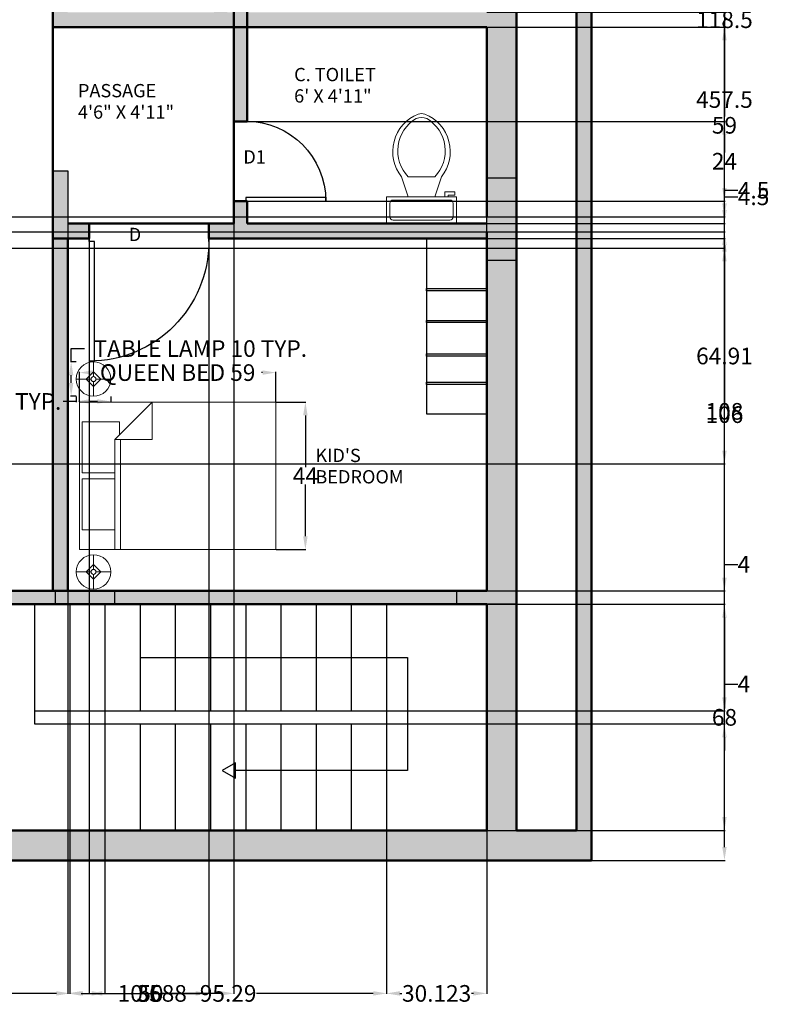
# Model space of a CAD drawing. Units: inches. Extents: x -12 to 887, y 330 to 874.
# Tile 6 of 9: x 662 to 887, y 330 to 626. Entities that reach past the tile are written whole.
import ezdxf

# ---------------------------------------------------------------- set-up
doc = ezdxf.new("R2010")
doc.units = ezdxf.units.IN
doc.header["$MEASUREMENT"] = 0
for name, color, linetype, lineweight in [('A-ANNO-DIMS', 2, 'Continuous', 18), ('A-ANNO-TEXT', 3, 'Continuous', 18), ('A-AREA-IDEN', 7, 'Continuous', 18), ('A-DOOR', 4, 'Continuous', 25), ('A-FLOR-FIXT', 8, 'Continuous', 18), ('A-FLOR-STRS', 3, 'Continuous', 25), ('A-FURN', 9, 'Continuous', 18), ('A-GLAZ', 4, 'Continuous', 25), ('A-WALL', 7, 'Continuous', 50), ('A-WALL-PATT', 5, 'Continuous', 13)]:
    doc.layers.add(name, color=color, linetype=linetype, lineweight=lineweight)
doc.styles.get("Standard").update_dxf_attribs({"font": 'arial.ttf'})
doc.dimstyles.get("Standard").update_dxf_attribs({"dimtxt": 5, "dimasz": 4, "dimexe": 0.18, "dimexo": 0.0625, "dimgap": 0.09, "dimtad": 0, "dimtih": 1, "dimtoh": 1, "dimdec": 1, "dimzin": 0, "dimdsep": 46, "dimlunit": 4, "dimtxsty": 'Standard', "dimcen": 0.09, "dimadec": 0, "dimazin": 0, "dimtfac": 1, "dimtdec": 1, "dimtofl": 0, "dimtmove": 0, "dimatfit": 3, "dimfxl": 1, "dimtolj": 1, "dimtzin": 0, "dimarcsym": 0})

# ---------------------------------------------------------------- blocks, each defined once
blk = doc.blocks.new('*U5')
for p, q in [((0, 0), (0, -6)), ((40, 0), (40, -6))]:
    blk.add_line(p, q)
blk.add_lwpolyline([(0, 0), (0, 40), (1.75, 40), (1.75, 0)], close=True)
blk.add_arc((0, 0), 40, 0, 90)
blk = doc.blocks.new('Bed - Queen')
for p, q in [((0, -80.00003), (0, 0)), ((0, 0), (59.99999, 0)), ((59.99999, 0), (59.99999, -80.00003)), ((7.99999, -1.2), (28.79998, -1.2)), ((7.99999, -14.4), (7.99999, -1.2)), ((28.79998, -1.2), (28.79998, -14.4)), ((31.19999, -1.2), (51.99999, -1.2)), ((31.19999, -14.4), (31.19999, -1.2)), ((51.99999, -1.2), (51.99999, -16.4)), ((0, -14.4), (44.8, -14.4)), ((59.99999, -29.6), (44.8, -14.4)), ((44.8, -14.4), (44.8, -29.6)), ((44.8, -16.8), (0, -16.8)), ((51.99999, -16.4), (46.79936, -16.4)), ((44.8, -29.6), (59.99999, -29.6)), ((59.99999, -80.00003), (0, -80.00003))]:
    blk.add_line(p, q)
blk = doc.blocks.new('Lamp - Table')
for p, q in [((0, 7), (0, 1)), ((-1, 0), (-7, 0)), ((0, 3), (-3, 0)), ((-3, 0), (0, -3)), ((3, 0), (0, 3)), ((0, -3), (3, 0)), ((1, 0), (7, 0)), ((0, -1), (0, -7))]:
    blk.add_line(p, q)
for radius in [7, 1]:
    blk.add_circle((0, 0), radius)
blk = doc.blocks.new('*U12')
for p, q in [((241.3, -152.4), (241.3, -50.8)), ((-254, -215.9), (-203.2, -215.9)), ((-254, -241.3), (-254, -215.9)), ((-203.2, -215.9), (-203.2, -203.2)), ((-177.8, -203.2), (-177.8, -241.3)), ((-101.6, -203.2), (-152.4, -355.6)), ((101.6, -203.2), (152.4, -355.6)), ((-177.8, -241.3), (-254, -241.3)), ((101.6, -355.6), (-101.6, -355.6))]:
    blk.add_line(p, q)
blk.add_lwpolyline([(266.7, -203.2), (266.7, 0), (-266.7, 0), (-266.7, -203.2)], close=True)
for points in [[(-241.3, -50.8), (-241.3, -152.4)], [(215.9, -25.4), (-215.9, -25.4)], [(-215.9, -177.8), (215.9, -177.8)]]:
    blk.add_lwpolyline(points)
for centre, radius, start, end in [((-219.1, -47.6), 22.5, 81.8699, 188.1301), ((219.1, -47.6), 22.5, 351.8699, 98.1301), ((-219.1, -155.6), 22.5, 171.8699, 278.1301), ((219.1, -155.6), 22.5, 261.8699, 8.1301), ((89.4, -548.1), 309.1, 141.46911, 247.97143), ((106.7, -554.2), 287.8, 136.36773, 238.94682), ((-89.4, -548.1), 309.1, 292.02843, 38.53071), ((-106.7, -554.2), 287.8, 301.05301, 43.63209), ((0, -708.1), 101.6, 245.73182, 294.26817), ((0, -736.6), 101.6, 254.86053, 285.13947)]:
    blk.add_arc(centre, radius, start, end)
blk = doc.blocks.new('*D18')
at = {"layer": 'A-ANNO-DIMS', "color": 0, "lineweight": -2, "transparency": 16777216}
for p, q in [((677.1, 523.03), (677.1, 527.03)), ((677.1, 527.03), (681.1, 527.03)), ((678.58, 523.03), (676.92, 523.03)), ((677.1, 516.69), (677.1, 519.03)), ((678.58, 512.69), (676.92, 512.69))]:
    blk.add_line(p, q, dxfattribs=at)
at = {"layer": 'A-ANNO-DIMS', "color": 0, "transparency": 16777216}
for points in [[(676.43, 519.03), (677.76, 519.03), (677.1, 523.03)], [(676.43, 516.69), (677.76, 516.69), (677.1, 512.69)]]:
    blk.add_solid(points, dxfattribs=at)
at = {"layer": 'Defpoints', "color": 0, "transparency": 16777216}
for p in [(677.1, 523.03), (678.65, 523.03), (678.65, 512.69)]:
    blk.add_point(p, dxfattribs=at)
at = {"layer": 'A-ANNO-DIMS', "color": 0, "transparency": 16777216, "insert": (715.93, 527.03), "char_height": 5, "attachment_point": 5}
blk.add_mtext('\\A1;TABLE LAMP 10 TYP.', dxfattribs=at)
blk = doc.blocks.new('*D19')
at = {"layer": 'A-ANNO-DIMS', "color": 0, "lineweight": -2, "transparency": 16777216}
for p, q in [((678.65, 512.63), (678.65, 510.96)), ((688.99, 512.63), (688.99, 510.96)), ((678.65, 511.14), (674.65, 511.14)), ((684.99, 511.14), (682.65, 511.14))]:
    blk.add_line(p, q, dxfattribs=at)
at = {"layer": 'A-ANNO-DIMS', "color": 0, "transparency": 16777216}
for points in [[(682.65, 511.8), (682.65, 510.47), (678.65, 511.14)], [(684.99, 511.8), (684.99, 510.47), (688.99, 511.14)]]:
    blk.add_solid(points, dxfattribs=at)
at = {"layer": 'Defpoints', "color": 0, "transparency": 16777216}
for p in [(678.65, 512.69), (688.99, 512.69), (678.65, 511.14)]:
    blk.add_point(p, dxfattribs=at)
at = {"layer": 'A-ANNO-DIMS', "color": 0, "transparency": 16777216, "insert": (662.62, 511.14), "char_height": 5, "attachment_point": 5}
blk.add_mtext('\\A1;10 TYP.', dxfattribs=at)
blk = doc.blocks.new('*D22')
at = {"layer": 'A-ANNO-DIMS', "color": 0, "lineweight": -2, "transparency": 16777216}
for p, q in [((679.56, 511.01), (679.56, 519.99)), ((683.56, 519.81), (683.91, 519.81)), ((734.67, 519.81), (734.33, 519.81)), ((738.67, 511.01), (738.67, 519.99))]:
    blk.add_line(p, q, dxfattribs=at)
at = {"layer": 'A-ANNO-DIMS', "color": 0, "transparency": 16777216}
for points in [[(683.56, 520.48), (683.56, 519.14), (679.56, 519.81)], [(734.67, 520.48), (734.67, 519.14), (738.67, 519.81)]]:
    blk.add_solid(points, dxfattribs=at)
at = {"layer": 'Defpoints', "color": 0, "transparency": 16777216}
for p in [(679.56, 519.81), (679.56, 510.94), (738.67, 510.94)]:
    blk.add_point(p, dxfattribs=at)
at = {"layer": 'A-ANNO-DIMS', "color": 0, "transparency": 16777216, "insert": (709.12, 519.81), "char_height": 5, "attachment_point": 5}
blk.add_mtext('\\A1;QUEEN BED 59', dxfattribs=at)
blk = doc.blocks.new('*D23')
at = {"layer": 'A-ANNO-DIMS', "color": 0, "lineweight": -2, "transparency": 16777216}
for p, q in [((738.74, 510.94), (747.72, 510.94)), ((747.54, 506.94), (747.54, 491.37)), ((747.54, 470.61), (747.54, 486.19)), ((738.74, 466.61), (747.72, 466.61))]:
    blk.add_line(p, q, dxfattribs=at)
at = {"layer": 'A-ANNO-DIMS', "color": 0, "transparency": 16777216}
for points in [[(746.87, 506.94), (748.21, 506.94), (747.54, 510.94)], [(746.87, 470.61), (748.21, 470.61), (747.54, 466.61)]]:
    blk.add_solid(points, dxfattribs=at)
at = {"layer": 'Defpoints', "color": 0, "transparency": 16777216}
for p in [(738.67, 510.94), (747.54, 510.94), (738.67, 466.61)]:
    blk.add_point(p, dxfattribs=at)
at = {"layer": 'A-ANNO-DIMS', "color": 0, "transparency": 16777216, "insert": (747.54, 488.78), "char_height": 5, "attachment_point": 5}
blk.add_mtext('\\A1;44', dxfattribs=at)
blk = doc.blocks.new('*D60')
at = {"layer": 'A-ANNO-DIMS', "color": 0, "lineweight": -2, "transparency": 16777216}
for p, q in [((383.99, 450.16), (873.75, 450.16)), ((873.57, 446.16), (873.57, 418.8)), ((873.57, 386.16), (873.57, 413.52)), ((383.99, 382.16), (873.75, 382.16))]:
    blk.add_line(p, q, dxfattribs=at)
at = {"layer": 'A-ANNO-DIMS', "color": 0, "transparency": 16777216}
for points in [[(872.9, 446.16), (874.24, 446.16), (873.57, 450.16)], [(872.9, 386.16), (874.24, 386.16), (873.57, 382.16)]]:
    blk.add_solid(points, dxfattribs=at)
at = {"layer": 'Defpoints', "color": 0, "transparency": 16777216}
for p in [(383.93, 450.16), (873.57, 450.16), (383.93, 382.16)]:
    blk.add_point(p, dxfattribs=at)
at = {"layer": 'A-ANNO-DIMS', "color": 0, "transparency": 16777216, "insert": (873.57, 416.16), "char_height": 5, "attachment_point": 5}
blk.add_mtext('\\A1;68', dxfattribs=at)
blk = doc.blocks.new('*D61')
at = {"layer": 'A-ANNO-DIMS', "color": 0, "lineweight": -2, "transparency": 16777216}
for p, q in [((873.57, 458.16), (873.57, 462.16)), ((873.57, 462.16), (877.57, 462.16)), ((383.99, 454.16), (873.75, 454.16)), ((383.99, 450.16), (873.75, 450.16)), ((873.57, 446.16), (873.57, 442.16))]:
    blk.add_line(p, q, dxfattribs=at)
at = {"layer": 'A-ANNO-DIMS', "color": 0, "transparency": 16777216}
for points in [[(872.9, 458.16), (874.24, 458.16), (873.57, 454.16)], [(872.9, 446.16), (874.24, 446.16), (873.57, 450.16)]]:
    blk.add_solid(points, dxfattribs=at)
at = {"layer": 'Defpoints', "color": 0, "transparency": 16777216}
for p in [(383.93, 454.16), (873.57, 454.16), (383.93, 450.16)]:
    blk.add_point(p, dxfattribs=at)
at = {"layer": 'A-ANNO-DIMS', "color": 0, "transparency": 16777216, "insert": (879.39, 462.16), "char_height": 5, "attachment_point": 5}
blk.add_mtext('\\A1;4', dxfattribs=at)
blk = doc.blocks.new('*D62')
at = {"layer": 'A-ANNO-DIMS', "color": 0, "lineweight": -2, "transparency": 16777216}
for p, q in [((383.99, 562.16), (873.75, 562.16)), ((873.57, 558.16), (873.57, 510.8)), ((873.57, 458.16), (873.57, 505.52)), ((383.99, 454.16), (873.75, 454.16))]:
    blk.add_line(p, q, dxfattribs=at)
at = {"layer": 'A-ANNO-DIMS', "color": 0, "transparency": 16777216}
for points in [[(872.9, 558.16), (874.24, 558.16), (873.57, 562.16)], [(872.9, 458.16), (874.24, 458.16), (873.57, 454.16)]]:
    blk.add_solid(points, dxfattribs=at)
at = {"layer": 'Defpoints', "color": 0, "transparency": 16777216}
for p in [(383.93, 562.16), (873.57, 562.16), (383.93, 454.16)]:
    blk.add_point(p, dxfattribs=at)
at = {"layer": 'A-ANNO-DIMS', "color": 0, "transparency": 16777216, "insert": (873.57, 508.16), "char_height": 5, "attachment_point": 5}
blk.add_mtext('\\A1;108', dxfattribs=at)
blk = doc.blocks.new('*D63')
at = {"layer": 'A-ANNO-DIMS', "color": 0, "lineweight": -2, "transparency": 16777216}
for p, q in [((873.57, 570.66), (873.57, 574.66)), ((873.57, 574.66), (877.57, 574.66)), ((383.99, 566.66), (873.75, 566.66)), ((383.99, 562.16), (873.75, 562.16)), ((873.57, 558.16), (873.57, 554.16))]:
    blk.add_line(p, q, dxfattribs=at)
at = {"layer": 'A-ANNO-DIMS', "color": 0, "transparency": 16777216}
for points in [[(872.9, 570.66), (874.24, 570.66), (873.57, 566.66)], [(872.9, 558.16), (874.24, 558.16), (873.57, 562.16)]]:
    blk.add_solid(points, dxfattribs=at)
at = {"layer": 'Defpoints', "color": 0, "transparency": 16777216}
for p in [(383.93, 566.66), (873.57, 566.66), (383.93, 562.16)]:
    blk.add_point(p, dxfattribs=at)
at = {"layer": 'A-ANNO-DIMS', "color": 0, "transparency": 16777216, "insert": (882.33, 574.66), "char_height": 5, "attachment_point": 5}
blk.add_mtext('\\A1;4.5', dxfattribs=at)
blk = doc.blocks.new('*D64')
at = {"layer": 'A-ANNO-DIMS', "color": 0, "lineweight": -2, "transparency": 16777216}
for p, q in [((383.99, 685.16), (873.75, 685.16)), ((873.57, 681.16), (873.57, 628.55)), ((873.57, 570.66), (873.57, 623.27)), ((383.99, 566.66), (873.75, 566.66))]:
    blk.add_line(p, q, dxfattribs=at)
at = {"layer": 'A-ANNO-DIMS', "color": 0, "transparency": 16777216}
for points in [[(872.9, 681.16), (874.24, 681.16), (873.57, 685.16)], [(872.9, 570.66), (874.24, 570.66), (873.57, 566.66)]]:
    blk.add_solid(points, dxfattribs=at)
at = {"layer": 'Defpoints', "color": 0, "transparency": 16777216}
for p in [(383.93, 685.16), (873.57, 685.16), (383.93, 566.66)]:
    blk.add_point(p, dxfattribs=at)
at = {"layer": 'A-ANNO-DIMS', "color": 0, "transparency": 16777216, "insert": (873.57, 625.91), "char_height": 5, "attachment_point": 5}
blk.add_mtext('\\A1;118.5', dxfattribs=at)
blk = doc.blocks.new('*D95')
at = {"layer": 'A-ANNO-DIMS', "color": 0, "lineweight": -2, "transparency": 16777216}
for p, q in [((493.07, 382.1), (493.07, 332.98)), ((676.66, 382.1), (676.66, 332.98)), ((497.07, 333.16), (576.57, 333.16)), ((672.66, 333.16), (593.15, 333.16))]:
    blk.add_line(p, q, dxfattribs=at)
at = {"layer": 'A-ANNO-DIMS', "color": 0, "transparency": 16777216}
for points in [[(497.07, 333.83), (497.07, 332.49), (493.07, 333.16)], [(672.66, 333.83), (672.66, 332.49), (676.66, 333.16)]]:
    blk.add_solid(points, dxfattribs=at)
at = {"layer": 'Defpoints', "color": 0, "transparency": 16777216}
for p in [(493.07, 382.16), (676.66, 382.16), (676.66, 333.16)]:
    blk.add_point(p, dxfattribs=at)
at = {"layer": 'A-ANNO-DIMS', "color": 0, "transparency": 16777216, "insert": (584.86, 333.16), "char_height": 5, "attachment_point": 5}
blk.add_mtext('\\A1;183.6', dxfattribs=at)
blk = doc.blocks.new('*D96')
at = {"layer": 'A-ANNO-DIMS', "color": 0, "lineweight": -2, "transparency": 16777216}
for p, q in [((676.66, 382.1), (676.66, 332.98)), ((771.95, 382.1), (771.95, 332.98)), ((680.66, 333.16), (715.77, 333.16)), ((767.95, 333.16), (732.83, 333.16))]:
    blk.add_line(p, q, dxfattribs=at)
at = {"layer": 'A-ANNO-DIMS', "color": 0, "transparency": 16777216}
for points in [[(680.66, 333.83), (680.66, 332.49), (676.66, 333.16)], [(767.95, 333.83), (767.95, 332.49), (771.95, 333.16)]]:
    blk.add_solid(points, dxfattribs=at)
at = {"layer": 'Defpoints', "color": 0, "transparency": 16777216}
for p in [(676.66, 382.16), (771.95, 382.16), (771.95, 333.16)]:
    blk.add_point(p, dxfattribs=at)
at = {"layer": 'A-ANNO-DIMS', "color": 0, "transparency": 16777216, "insert": (724.3, 333.16), "char_height": 5, "attachment_point": 5}
blk.add_mtext('\\A1;95.29', dxfattribs=at)
blk = doc.blocks.new('*D97')
at = {"layer": 'A-ANNO-DIMS', "color": 0, "lineweight": -2, "transparency": 16777216}
for p, q in [((771.95, 382.1), (771.95, 332.98)), ((802.07, 382.1), (802.07, 332.98)), ((775.95, 333.16), (776.54, 333.16)), ((798.07, 333.16), (797.47, 333.16))]:
    blk.add_line(p, q, dxfattribs=at)
at = {"layer": 'A-ANNO-DIMS', "color": 0, "transparency": 16777216}
for points in [[(775.95, 333.83), (775.95, 332.49), (771.95, 333.16)], [(798.07, 333.83), (798.07, 332.49), (802.07, 333.16)]]:
    blk.add_solid(points, dxfattribs=at)
at = {"layer": 'Defpoints', "color": 0, "transparency": 16777216}
for p in [(771.95, 382.16), (802.07, 382.16), (802.07, 333.16)]:
    blk.add_point(p, dxfattribs=at)
at = {"layer": 'A-ANNO-DIMS', "color": 0, "transparency": 16777216, "insert": (787.01, 333.16), "char_height": 5, "attachment_point": 5}
blk.add_mtext('\\A1;30.123', dxfattribs=at)
blk = doc.blocks.new('*D98')
at = {"layer": 'A-ANNO-DIMS', "color": 0, "lineweight": -2, "transparency": 16777216}
for p, q in [((460.13, 830.66), (873.75, 830.66)), ((873.57, 826.66), (873.57, 604.54)), ((873.57, 377.16), (873.57, 599.28)), ((460.13, 373.16), (873.75, 373.16))]:
    blk.add_line(p, q, dxfattribs=at)
at = {"layer": 'A-ANNO-DIMS', "color": 0, "transparency": 16777216}
for points in [[(872.9, 826.66), (874.24, 826.66), (873.57, 830.66)], [(872.9, 377.16), (874.24, 377.16), (873.57, 373.16)]]:
    blk.add_solid(points, dxfattribs=at)
at = {"layer": 'Defpoints', "color": 0, "transparency": 16777216}
for p in [(460.07, 830.66), (873.57, 830.66), (460.07, 373.16)]:
    blk.add_point(p, dxfattribs=at)
at = {"layer": 'A-ANNO-DIMS', "color": 0, "transparency": 16777216, "insert": (873.57, 601.91), "char_height": 5, "attachment_point": 5}
blk.add_mtext('\\A1;457.5', dxfattribs=at)
blk = doc.blocks.new('*D104')
at = {"layer": 'A-ANNO-DIMS', "color": 0, "lineweight": -2, "transparency": 16777216}
for p, q in [((802.13, 450.16), (873.75, 450.16)), ((873.57, 446.16), (873.57, 418.8)), ((873.57, 386.16), (873.57, 413.52)), ((802.13, 382.16), (873.75, 382.16))]:
    blk.add_line(p, q, dxfattribs=at)
at = {"layer": 'A-ANNO-DIMS', "color": 0, "transparency": 16777216}
for points in [[(872.9, 446.16), (874.24, 446.16), (873.57, 450.16)], [(872.9, 386.16), (874.24, 386.16), (873.57, 382.16)]]:
    blk.add_solid(points, dxfattribs=at)
at = {"layer": 'Defpoints', "color": 0, "transparency": 16777216}
for p in [(802.07, 450.16), (873.57, 450.16), (802.07, 382.16)]:
    blk.add_point(p, dxfattribs=at)
at = {"layer": 'A-ANNO-DIMS', "color": 0, "transparency": 16777216, "insert": (873.57, 416.16), "char_height": 5, "attachment_point": 5}
blk.add_mtext('\\A1;68', dxfattribs=at)
blk = doc.blocks.new('*D105')
at = {"layer": 'A-ANNO-DIMS', "color": 0, "lineweight": -2, "transparency": 16777216}
for p, q in [((873.57, 458.16), (873.57, 462.16)), ((873.57, 462.16), (877.57, 462.16)), ((802.13, 454.16), (873.75, 454.16)), ((802.13, 450.16), (873.75, 450.16)), ((873.57, 446.16), (873.57, 442.16))]:
    blk.add_line(p, q, dxfattribs=at)
at = {"layer": 'A-ANNO-DIMS', "color": 0, "transparency": 16777216}
for points in [[(872.9, 458.16), (874.24, 458.16), (873.57, 454.16)], [(872.9, 446.16), (874.24, 446.16), (873.57, 450.16)]]:
    blk.add_solid(points, dxfattribs=at)
at = {"layer": 'Defpoints', "color": 0, "transparency": 16777216}
for p in [(802.07, 454.16), (873.57, 454.16), (802.07, 450.16)]:
    blk.add_point(p, dxfattribs=at)
at = {"layer": 'A-ANNO-DIMS', "color": 0, "transparency": 16777216, "insert": (879.39, 462.16), "char_height": 5, "attachment_point": 5}
blk.add_mtext('\\A1;4', dxfattribs=at)
blk = doc.blocks.new('*D106')
at = {"layer": 'A-ANNO-DIMS', "color": 0, "lineweight": -2, "transparency": 16777216}
for p, q in [((802.13, 560.16), (873.75, 560.16)), ((873.57, 556.16), (873.57, 509.8)), ((873.57, 458.16), (873.57, 504.52)), ((802.13, 454.16), (873.75, 454.16))]:
    blk.add_line(p, q, dxfattribs=at)
at = {"layer": 'A-ANNO-DIMS', "color": 0, "transparency": 16777216}
for points in [[(872.9, 556.16), (874.24, 556.16), (873.57, 560.16)], [(872.9, 458.16), (874.24, 458.16), (873.57, 454.16)]]:
    blk.add_solid(points, dxfattribs=at)
at = {"layer": 'Defpoints', "color": 0, "transparency": 16777216}
for p in [(802.07, 560.16), (873.57, 560.16), (802.07, 454.16)]:
    blk.add_point(p, dxfattribs=at)
at = {"layer": 'A-ANNO-DIMS', "color": 0, "transparency": 16777216, "insert": (873.57, 507.16), "char_height": 5, "attachment_point": 5}
blk.add_mtext('\\A1;106', dxfattribs=at)
blk = doc.blocks.new('*D107')
at = {"layer": 'A-ANNO-DIMS', "color": 0, "lineweight": -2, "transparency": 16777216}
for p, q in [((873.57, 568.66), (873.57, 572.66)), ((873.57, 572.66), (877.57, 572.66)), ((802.13, 564.66), (873.75, 564.66)), ((802.13, 560.16), (873.75, 560.16)), ((873.57, 556.16), (873.57, 552.16))]:
    blk.add_line(p, q, dxfattribs=at)
at = {"layer": 'A-ANNO-DIMS', "color": 0, "transparency": 16777216}
for points in [[(872.9, 568.66), (874.24, 568.66), (873.57, 564.66)], [(872.9, 556.16), (874.24, 556.16), (873.57, 560.16)]]:
    blk.add_solid(points, dxfattribs=at)
at = {"layer": 'Defpoints', "color": 0, "transparency": 16777216}
for p in [(802.07, 564.66), (873.57, 564.66), (802.07, 560.16)]:
    blk.add_point(p, dxfattribs=at)
at = {"layer": 'A-ANNO-DIMS', "color": 0, "transparency": 16777216, "insert": (882.33, 572.66), "char_height": 5, "attachment_point": 5}
blk.add_mtext('\\A1;4.5', dxfattribs=at)
blk = doc.blocks.new('*D108')
at = {"layer": 'A-ANNO-DIMS', "color": 0, "lineweight": -2, "transparency": 16777216}
for p, q in [((802.13, 623.66), (873.75, 623.66)), ((873.57, 619.66), (873.57, 596.8)), ((873.57, 568.66), (873.57, 591.52)), ((802.13, 564.66), (873.75, 564.66))]:
    blk.add_line(p, q, dxfattribs=at)
at = {"layer": 'A-ANNO-DIMS', "color": 0, "transparency": 16777216}
for points in [[(872.9, 619.66), (874.24, 619.66), (873.57, 623.66)], [(872.9, 568.66), (874.24, 568.66), (873.57, 564.66)]]:
    blk.add_solid(points, dxfattribs=at)
at = {"layer": 'Defpoints', "color": 0, "transparency": 16777216}
for p in [(802.07, 623.66), (873.57, 623.66), (802.07, 564.66)]:
    blk.add_point(p, dxfattribs=at)
at = {"layer": 'A-ANNO-DIMS', "color": 0, "transparency": 16777216, "insert": (873.57, 594.16), "char_height": 5, "attachment_point": 5}
blk.add_mtext('\\A1;59', dxfattribs=at)
blk = doc.blocks.new('*D109')
at = {"layer": 'A-ANNO-DIMS', "color": 0, "lineweight": -2, "transparency": 16777216}
for p, q in [((873.57, 632.16), (873.57, 636.16)), ((873.57, 636.16), (877.57, 636.16)), ((802.13, 628.16), (873.75, 628.16)), ((802.13, 623.66), (873.75, 623.66)), ((873.57, 619.66), (873.57, 615.66))]:
    blk.add_line(p, q, dxfattribs=at)
at = {"layer": 'A-ANNO-DIMS', "color": 0, "transparency": 16777216}
for points in [[(872.9, 632.16), (874.24, 632.16), (873.57, 628.16)], [(872.9, 619.66), (874.24, 619.66), (873.57, 623.66)]]:
    blk.add_solid(points, dxfattribs=at)
at = {"layer": 'Defpoints', "color": 0, "transparency": 16777216}
for p in [(802.07, 628.16), (873.57, 628.16), (802.07, 623.66)]:
    blk.add_point(p, dxfattribs=at)
at = {"layer": 'A-ANNO-DIMS', "color": 0, "transparency": 16777216, "insert": (882.33, 636.16), "char_height": 5, "attachment_point": 5}
blk.add_mtext('\\A1;4.5', dxfattribs=at)
blk = doc.blocks.new('*D115')
at = {"layer": 'A-ANNO-DIMS', "color": 0, "lineweight": -2, "transparency": 16777216}
for p, q in [((676.07, 564.6), (676.07, 332.98)), ((726.07, 564.6), (726.07, 332.98)), ((680.07, 333.16), (697.41, 333.16)), ((722.07, 333.16), (704.73, 333.16))]:
    blk.add_line(p, q, dxfattribs=at)
at = {"layer": 'A-ANNO-DIMS', "color": 0, "transparency": 16777216}
for points in [[(680.07, 333.83), (680.07, 332.49), (676.07, 333.16)], [(722.07, 333.83), (722.07, 332.49), (726.07, 333.16)]]:
    blk.add_solid(points, dxfattribs=at)
at = {"layer": 'Defpoints', "color": 0, "transparency": 16777216}
for p in [(676.07, 564.66), (726.07, 564.66), (726.07, 333.16)]:
    blk.add_point(p, dxfattribs=at)
at = {"layer": 'A-ANNO-DIMS', "color": 0, "transparency": 16777216, "insert": (701.07, 333.16), "char_height": 5, "attachment_point": 5}
blk.add_mtext('\\A1;50', dxfattribs=at)
blk = doc.blocks.new('*D118')
at = {"layer": 'A-ANNO-DIMS', "color": 0, "lineweight": -2, "transparency": 16777216}
for p, q in [((873.57, 422.16), (873.57, 426.16)), ((873.57, 426.16), (877.57, 426.16)), ((666.13, 418.16), (873.75, 418.16)), ((666.13, 414.16), (873.75, 414.16)), ((873.57, 410.16), (873.57, 406.16))]:
    blk.add_line(p, q, dxfattribs=at)
at = {"layer": 'A-ANNO-DIMS', "color": 0, "transparency": 16777216}
for points in [[(872.9, 422.16), (874.24, 422.16), (873.57, 418.16)], [(872.9, 410.16), (874.24, 410.16), (873.57, 414.16)]]:
    blk.add_solid(points, dxfattribs=at)
at = {"layer": 'Defpoints', "color": 0, "transparency": 16777216}
for p in [(666.07, 418.16), (873.57, 418.16), (666.07, 414.16)]:
    blk.add_point(p, dxfattribs=at)
at = {"layer": 'A-ANNO-DIMS', "color": 0, "transparency": 16777216, "insert": (879.39, 426.16), "char_height": 5, "attachment_point": 5}
blk.add_mtext('\\A1;4', dxfattribs=at)
blk = doc.blocks.new('*D119')
at = {"layer": 'A-ANNO-DIMS', "color": 0, "lineweight": -2, "transparency": 16777216}
for p, q in [((676.66, 418.1), (676.66, 332.98)), ((687.24, 418.1), (687.24, 332.98)), ((680.66, 333.16), (683.24, 333.16)), ((687.24, 333.16), (691.24, 333.16))]:
    blk.add_line(p, q, dxfattribs=at)
at = {"layer": 'A-ANNO-DIMS', "color": 0, "transparency": 16777216}
for points in [[(680.66, 333.83), (680.66, 332.49), (676.66, 333.16)], [(683.24, 333.83), (683.24, 332.49), (687.24, 333.16)]]:
    blk.add_solid(points, dxfattribs=at)
at = {"layer": 'Defpoints', "color": 0, "transparency": 16777216}
for p in [(676.66, 418.16), (687.24, 418.16), (687.24, 333.16)]:
    blk.add_point(p, dxfattribs=at)
at = {"layer": 'A-ANNO-DIMS', "color": 0, "transparency": 16777216, "insert": (701.48, 333.16), "char_height": 5, "attachment_point": 5}
blk.add_mtext('\\A1;10.588', dxfattribs=at)
blk = doc.blocks.new('*D124')
at = {"layer": 'A-ANNO-DIMS', "color": 0, "lineweight": -2, "transparency": 16777216}
for p, q in [((682.52, 564.6), (682.52, 332.98)), ((718.52, 564.6), (718.52, 332.98)), ((686.52, 333.16), (696.85, 333.16)), ((714.52, 333.16), (704.19, 333.16))]:
    blk.add_line(p, q, dxfattribs=at)
at = {"layer": 'A-ANNO-DIMS', "color": 0, "transparency": 16777216}
for points in [[(686.52, 333.83), (686.52, 332.49), (682.52, 333.16)], [(714.52, 333.83), (714.52, 332.49), (718.52, 333.16)]]:
    blk.add_solid(points, dxfattribs=at)
at = {"layer": 'Defpoints', "color": 0, "transparency": 16777216}
for p in [(682.52, 564.66), (718.52, 564.66), (718.52, 333.16)]:
    blk.add_point(p, dxfattribs=at)
at = {"layer": 'A-ANNO-DIMS', "color": 0, "transparency": 16777216, "insert": (700.52, 333.16), "char_height": 5, "attachment_point": 5}
blk.add_mtext('\\A1;36', dxfattribs=at)
blk = doc.blocks.new('*D125')
at = {"layer": 'A-ANNO-DIMS', "color": 0, "lineweight": -2, "transparency": 16777216}
for p, q in [((726.13, 595.35), (873.75, 595.35)), ((873.57, 591.35), (873.57, 585.95)), ((873.57, 575.35), (873.57, 580.75)), ((726.13, 571.35), (873.75, 571.35))]:
    blk.add_line(p, q, dxfattribs=at)
at = {"layer": 'A-ANNO-DIMS', "color": 0, "transparency": 16777216}
for points in [[(872.9, 591.35), (874.24, 591.35), (873.57, 595.35)], [(872.9, 575.35), (874.24, 575.35), (873.57, 571.35)]]:
    blk.add_solid(points, dxfattribs=at)
at = {"layer": 'Defpoints', "color": 0, "transparency": 16777216}
for p in [(726.07, 595.35), (726.07, 571.35), (873.57, 571.35)]:
    blk.add_point(p, dxfattribs=at)
at = {"layer": 'A-ANNO-DIMS', "color": 0, "transparency": 16777216, "insert": (873.57, 583.35), "char_height": 5, "attachment_point": 5}
blk.add_mtext('\\A1;24', dxfattribs=at)
blk = doc.blocks.new('*D129')
at = {"layer": 'A-ANNO-DIMS', "color": 0, "lineweight": -2, "transparency": 16777216}
for p, q in [((488.63, 557.26), (873.75, 557.26)), ((873.57, 553.26), (873.57, 527.44)), ((873.57, 496.34), (873.57, 522.16)), ((488.63, 492.34), (873.75, 492.34))]:
    blk.add_line(p, q, dxfattribs=at)
at = {"layer": 'A-ANNO-DIMS', "color": 0, "transparency": 16777216}
for points in [[(872.9, 553.26), (874.24, 553.26), (873.57, 557.26)], [(872.9, 496.34), (874.24, 496.34), (873.57, 492.34)]]:
    blk.add_solid(points, dxfattribs=at)
at = {"layer": 'Defpoints', "color": 0, "transparency": 16777216}
for p in [(488.57, 557.26), (488.57, 492.34), (873.57, 492.34)]:
    blk.add_point(p, dxfattribs=at)
at = {"layer": 'A-ANNO-DIMS', "color": 0, "transparency": 16777216, "insert": (873.57, 524.8), "char_height": 5, "attachment_point": 5}
blk.add_mtext('\\A1;64.91', dxfattribs=at)

msp = doc.modelspace()

# ---------------------------------------------------------------- hatches: boundary and pattern name
at = {"layer": 'A-WALL-PATT'}
h = msp.add_hatch(color=256, dxfattribs=at)
h.dxf.hatch_style = 1
h.paths.add_polyline_path([(94.575, 830.6611), (67.3199, 830.6611), (67.3199, 821.6611), (70.4263, 821.6611), (79.4263, 821.6611), (94.575, 821.6611)])
h.paths.add_polyline_path([(288.8031, 830.6611), (257.9263, 830.6611), (253.4263, 830.6611), (253.4263, 821.6611), (288.8031, 821.6611)])
h.paths.add_polyline_path([(74.9263, 696.9265), (70.4263, 696.9265), (70.4263, 678.4656), (74.9263, 678.4656)])
h.paths.add_polyline_path([(74.9263, 584.8756), (70.4263, 584.8756), (70.4263, 562.1611), (74.9263, 562.1611)])
h.paths.add_polyline_path([(135.5357, 566.6611), (122.6994, 566.6611), (122.6994, 562.1611), (135.5357, 562.1611)])
h.paths.add_polyline_path([(257.9263, 579.1607), (253.4263, 579.1607), (253.4263, 562.1611), (257.9263, 562.1611)])
h.paths.add_polyline_path([(272.0195, 454.1611), (254.2006, 454.1611), (254.2006, 450.1611), (272.0195, 450.1611)])
h.paths.add_polyline_path([(392.9263, 454.1611), (374.959, 454.1611), (374.959, 450.1611), (383.9263, 450.1611), (392.9263, 450.1611)])
h.paths.add_polyline_path([(493.0683, 466.4171), (488.5683, 466.4171), (488.5683, 450.1611), (493.0683, 450.1611)])
h.paths.add_polyline_path([(568.6302, 454.1611), (555.938, 454.1611), (555.938, 450.1611), (568.6302, 450.1611)])
h.paths.add_polyline_path([(493.0683, 594.9471), (488.5683, 594.9471), (488.5683, 569.5862), (493.0683, 569.5862)])
h.paths.add_polyline_path([(690.1615, 454.1611), (672.3426, 454.1611), (672.3426, 450.1611), (690.1615, 450.1611)])
h.paths.add_polyline_path([(811.0683, 454.1611), (793.101, 454.1611), (793.101, 450.1611), (802.0683, 450.1611), (811.0683, 450.1611)])
h.paths.add_polyline_path([(811.0683, 578.3606), (802.0683, 578.3606), (802.0683, 566.6611), (802.0683, 553.5254), (811.0683, 553.5254)])
h.paths.add_polyline_path([(811.0683, 701.6611), (802.0683, 701.6611), (802.0683, 689.9616), (802.0683, 676.8259), (811.0683, 676.8259)])
h.paths.add_polyline_path([(811.0683, 830.6611), (782.165, 830.6611), (782.165, 821.6611), (802.0683, 821.6611), (811.0683, 821.6611)])
h.paths.add_polyline_path([(706.9451, 830.6611), (671.5683, 830.6611), (671.5683, 821.6611), (706.9451, 821.6611)])
h.paths.add_polyline_path([(512.717, 830.6611), (485.4619, 830.6611), (485.4619, 821.6611), (488.5683, 821.6611), (512.717, 821.6611)])
h.paths.add_polyline_path([(392.9263, 697.8668), (383.9263, 697.8668), (383.9263, 689.6611), (383.9263, 676.5034), (392.9263, 676.5034)])
h.paths.add_polyline_path([(392.9263, 830.6611), (364.023, 830.6611), (364.023, 821.7357), (392.9263, 821.7357)])
h.paths.add_polyline_path([(392.9263, 619.0434), (383.9263, 619.0434), (383.9263, 588.7499), (392.9263, 588.7499)])
h.paths.add_polyline_path([(392.9263, 578.3606), (383.9263, 578.3606), (383.9263, 566.6611), (383.9263, 553.5254), (392.9263, 553.5254)])
h.paths.add_polyline_path([(257.9263, 699.8547), (253.4263, 699.8547), (253.4263, 697.1611), (253.4263, 677.338), (257.9263, 677.338)])
h.paths.add_polyline_path([(493.0683, 714.3785), (488.5683, 714.3785), (488.5683, 689.6611), (493.0683, 689.6611)])
h.paths.add_polyline_path([(74.9263, 491.4191), (70.4263, 491.4191), (70.4263, 480.7097), (74.9263, 480.7097)])
h = msp.add_hatch(color=256, dxfattribs=at)
h.dxf.hatch_style = 1
h.paths.add_polyline_path([(671.5683, 830.6611), (512.717, 830.6611), (512.717, 821.6611), (617.0825, 821.6611), (617.0825, 797.5825), (617.0787, 783.3094), (621.5683, 783.3094), (621.5683, 821.6611), (671.5683, 821.6611)], flags=17)
h.paths.add_polyline_path([(833.5683, 830.6611), (811.0683, 830.6611), (811.0683, 821.6611), (829.0683, 821.6611), (829.0683, 701.6611), (829.0683, 382.1611), (811.0683, 382.1611), (811.0683, 450.1611), (802.0683, 450.1611), (802.0683, 382.1611), (671.5683, 382.1611), (464.5683, 382.1611), (464.5683, 821.6611), (460.0683, 821.6611), (460.0683, 373.1611), (671.5683, 373.1611), (833.5683, 373.1611)])
h.paths.add_polyline_path([(493.0683, 728.8273), (488.5683, 728.8273), (488.5683, 714.3785), (493.0683, 714.3785)], flags=17)
h.paths.add_polyline_path([(493.0683, 821.6611), (488.5683, 821.6611), (488.5683, 781.3634), (493.0683, 781.3634)], flags=17)
h = msp.add_hatch(color=256, dxfattribs=at)
h.dxf.hatch_style = 1
h.paths.add_polyline_path([(485.4619, 830.6611), (460.0683, 830.6611), (460.0683, 373.1611), (833.5683, 373.1611), (833.5683, 830.6611), (811.0683, 830.6611), (811.0683, 821.6611), (829.0683, 821.6611), (829.0683, 701.6611), (829.0683, 382.1611), (811.0683, 382.1611), (811.0683, 450.1611), (802.0683, 450.1611), (802.0683, 382.1611), (671.5683, 382.1611), (464.5683, 382.1611), (464.5683, 821.6611), (485.4619, 821.6611)])
h = msp.add_hatch(color=256, dxfattribs=at)
h.dxf.hatch_style = 1
h.paths.add_polyline_path([(671.5683, 749.6611), (621.5683, 749.6611), (621.5683, 759.3094), (620.6653, 759.3094), (617.0683, 759.3094), (617.0683, 745.1611), (671.5683, 745.1611)])
h.paths.add_polyline_path([(676.0683, 821.6611), (671.5683, 821.6611), (671.5683, 736.2424), (676.0683, 736.2424)])
h.paths.add_polyline_path([(782.165, 830.6611), (706.9451, 830.6611), (706.9451, 821.6611), (782.165, 821.6611)])
h.paths.add_polyline_path([(811.0683, 553.5254), (802.0683, 553.5254), (802.0683, 507.4529), (802.0683, 454.1611), (811.0683, 454.1611)])
h.paths.add_polyline_path([(793.101, 454.1611), (690.1615, 454.1611), (690.1615, 450.1611), (793.101, 450.1611)])
h.paths.add_polyline_path([(672.3426, 454.1611), (656.7304, 454.1611), (656.7304, 450.1611), (672.3426, 450.1611)])
h.paths.add_polyline_path([(582.6585, 454.1611), (568.6302, 454.1611), (568.6302, 450.1611), (582.6585, 450.1611)])
h.paths.add_polyline_path([(555.938, 454.1611), (554.2565, 454.1611), (554.2565, 452.8628), (554.2565, 450.1611), (555.938, 450.1611)])
h.paths.add_polyline_path([(518.2335, 452.8628), (518.2335, 454.1611), (493.0683, 454.1611), (493.0683, 450.1611), (518.2335, 450.1611)])
h.paths.add_polyline_path([(493.0683, 450.1611), (488.5683, 450.1611), (488.5683, 382.1611), (493.0683, 382.1611)])
h.paths.add_polyline_path([(493.0683, 492.3446), (488.5683, 492.3446), (488.5683, 466.4171), (493.0683, 466.4171)])
h.paths.add_polyline_path([(493.0683, 569.5862), (488.5683, 569.5862), (488.5683, 557.2595), (493.0683, 557.2595)])
h.paths.add_polyline_path([(493.0683, 689.6611), (488.5683, 689.6611), (488.5683, 594.9471), (493.0683, 594.9471)])
h.paths.add_polyline_path([(676.0683, 700.2227), (671.5683, 700.2227), (671.5683, 669.5589), (676.0683, 669.5589)])
h.paths.add_polyline_path([(739.0683, 689.6611), (676.0683, 689.6611), (676.0683, 685.1611), (739.0683, 685.1611)])
h.paths.add_polyline_path([(802.0683, 689.6611), (763.0683, 689.6611), (763.0683, 686.0698), (763.0683, 685.1611), (802.0683, 685.1611)])
h.paths.add_polyline_path([(811.0683, 821.6611), (802.0683, 821.6611), (802.0683, 756.0738), (811.0683, 756.0738)])
h.paths.add_polyline_path([(811.0683, 707.8935), (802.0683, 707.8935), (802.0683, 701.6611), (811.0683, 701.6611)])
h.paths.add_polyline_path([(811.0683, 676.8259), (802.0683, 676.8259), (802.0683, 628.1611), (730.0683, 628.1611), (730.0683, 623.6611), (802.0683, 623.6611), (802.0683, 578.3606), (811.0683, 578.3606)])
h.paths.add_polyline_path([(730.0683, 685.1611), (726.0683, 685.1611), (726.0683, 628.1611), (730.0683, 628.1611)])
h.paths.add_polyline_path([(724.0683, 685.1611), (720.0683, 685.1611), (720.0683, 628.1611), (724.0683, 628.1611)])
h.paths.add_polyline_path([(726.0683, 628.1611), (676.0683, 628.1611), (676.0683, 633.7662), (674.2492, 633.7662), (671.5683, 633.7662), (671.5683, 623.6611), (726.0683, 623.6611)])
h.paths.add_polyline_path([(730.0683, 628.1611), (726.0683, 628.1611), (726.0683, 623.6611), (730.0683, 623.6611)])
h.paths.add_polyline_path([(730.0683, 623.6611), (726.0683, 623.6611), (726.0683, 595.3822), (729.6731, 595.3822, -0.00411226), (730.0683, 595.379)])
h.paths.add_polyline_path([(802.0683, 564.6611), (730.0683, 564.6611), (730.0683, 571.3507), (729.6731, 571.3507), (726.0683, 571.3507), (726.0683, 564.6611), (718.522, 564.6611), (718.522, 560.1611), (802.0683, 560.1611)])
h.paths.add_polyline_path([(676.0683, 580.4772), (671.5683, 580.4772), (671.5683, 560.1611), (676.0683, 560.1611)])
h.paths.add_polyline_path([(682.5176, 564.6611), (676.0683, 564.6611), (676.0683, 560.1611), (682.5176, 560.1611)])
h.paths.add_polyline_path([(676.0683, 560.1611), (671.5683, 560.1611), (671.5683, 454.1611), (672.3426, 454.1611), (676.0683, 454.1611)])

# ---------------------------------------------------------------- linework, layer by layer
at = {"layer": 'A-FLOR-STRS'}
for p, q in [((666.0683, 450.1611), (666.0683, 414.1611)), ((676.656, 450.1611), (676.656, 418.1611)), ((687.2437, 450.1611), (687.2437, 418.1611)), ((697.8314, 450.1611), (697.8314, 418.1611)), ((708.419, 450.1611), (708.419, 418.1611)), ((719.0067, 450.1611), (719.0067, 418.1611)), ((729.5944, 450.1611), (729.5944, 418.1611)), ((740.182, 450.1611), (740.182, 418.1611)), ((750.7697, 450.1611), (750.7697, 418.1611)), ((761.3574, 450.1611), (761.3574, 418.1611)), ((771.9451, 450.1611), (771.9451, 418.1611)), ((697.8314, 434.1611), (778.2474, 434.1611)), ((778.2474, 434.1611), (778.2474, 400.1611)), ((666.0683, 418.1611), (771.9451, 418.1611)), ((771.9451, 418.1611), (771.9451, 382.1611)), ((666.0683, 414.1611), (771.9451, 414.1611)), ((676.656, 414.1611), (676.656, 382.1611)), ((687.2437, 414.1611), (687.2437, 382.1611)), ((697.8314, 414.1611), (697.8314, 382.1611)), ((708.419, 414.1611), (708.419, 382.1611)), ((719.0067, 414.1611), (719.0067, 382.1611)), ((729.5944, 414.1611), (729.5944, 382.1611)), ((740.182, 414.1611), (740.182, 382.1611)), ((750.7697, 414.1611), (750.7697, 382.1611)), ((761.3574, 414.1611), (761.3574, 382.1611)), ((726.5408, 402.5244), (722.5497, 400.1611)), ((722.5497, 400.1611), (726.5408, 397.8475)), ((726.5408, 400.1611), (726.5408, 402.5244)), ((778.2474, 400.1611), (726.5408, 400.1611)), ((726.5408, 397.8475), (726.5408, 400.1611))]:
    msp.add_line(p, q, dxfattribs=at)
for points in [[(802.0683, 560.1611), (783.9673, 560.1611), (783.9673, 507.4529), (802.0683, 507.4529)], [(783.9673, 545.1004), (802.0683, 545.1004), (802.0683, 544.4154), (783.9673, 544.4154)], [(783.9673, 535.5054), (802.0683, 535.5054), (802.0683, 534.8203), (783.9673, 534.8203)], [(783.9673, 525.4423), (802.0683, 525.4423), (802.0683, 524.7572), (783.9673, 524.7572)], [(783.9673, 516.9003), (802.0683, 516.9003), (802.0683, 516.2152), (783.9673, 516.2152)]]:
    msp.add_lwpolyline(points, close=True, dxfattribs=at)
at = {"layer": 'A-GLAZ'}
for points in [[(676.0683, 560.1611), (671.5683, 560.1611), (671.5683, 580.4772), (676.0683, 580.4772)], [(672.3426, 454.1611), (690.1615, 454.1611), (690.1615, 450.1611), (672.3426, 450.1611)], [(793.101, 454.1611), (811.0683, 454.1611), (811.0683, 450.1611), (793.101, 450.1611)]]:
    msp.add_lwpolyline(points, close=True, dxfattribs=at)
msp.add_lwpolyline([(802.0683, 566.6611), (802.0683, 578.3606), (811.0683, 578.3606), (811.0683, 553.5254), (802.0683, 553.5254), (802.0683, 566.6611)], dxfattribs=at)
at = {"layer": 'A-WALL'}
for p, q in [((671.5683, 830.6611), (671.5683, 584.9963)), ((833.5683, 830.6611), (833.5683, 373.1611)), ((811.0683, 821.6611), (811.0683, 382.1611)), ((829.0683, 701.6611), (829.0683, 382.1611)), ((726.0683, 685.1611), (726.0683, 564.6611)), ((730.0683, 685.1611), (730.0683, 595.3507)), ((671.5683, 623.6611), (802.0683, 623.6611)), ((802.0683, 623.6611), (802.0683, 566.6611)), ((802.0683, 623.6611), (802.0683, 577.1611)), ((730.0683, 595.3507), (726.0683, 595.3507)), ((671.5683, 584.9963), (671.5683, 454.1611)), ((726.0683, 571.3507), (730.0683, 571.3507)), ((730.0683, 571.3507), (730.0683, 564.6611)), ((676.0683, 564.6611), (726.0683, 564.6611)), ((682.5176, 564.6611), (682.5176, 560.1611)), ((718.5176, 560.1611), (718.5176, 564.6611)), ((730.0683, 564.6611), (802.0683, 564.6611)), ((671.5683, 560.1611), (682.5176, 560.1611)), ((676.0683, 560.1611), (676.0683, 454.1611)), ((718.5176, 560.1611), (802.0683, 560.1611)), ((802.0683, 562.1611), (802.0683, 454.1611)), ((554.245, 454.1611), (802.0683, 454.1611)), ((488.5683, 450.1611), (802.0683, 450.1611)), ((802.0683, 450.1611), (802.0683, 382.1611)), ((464.5683, 382.1611), (671.5683, 382.1611)), ((671.5683, 382.1611), (802.0683, 382.1611)), ((811.0683, 382.1611), (829.0683, 382.1611)), ((460.0683, 373.1611), (833.5683, 373.1611))]:
    msp.add_line(p, q, dxfattribs=at)

# ---------------------------------------------------------------- block references
at = {"layer": 'A-DOOR'}
for p, xscale, yscale, zscale, rotation in [((729.6731, 571.3507), -0.6007875453040183, 0.6007875453040183, 0.6007875453040183, 270), ((682.5176, 559.2604), -0.9001099302617062, 0.9001099302617062, 0.9001099302617062, 180)]:
    msp.add_blockref('*U5', p, dxfattribs=dict(at, xscale=xscale, yscale=yscale, zscale=zscale, rotation=rotation))
at = {"layer": 'A-FLOR-FIXT', "xscale": 0.0393700787401575, "yscale": 0.0393700787401575, "zscale": 0.0393700787401575, "rotation": 180}
msp.add_blockref('*U12', (782.455, 564.6611), dxfattribs=at)
at = {"layer": 'A-FURN', "xscale": 0.7388583925740742, "yscale": 0.7388583925740742, "zscale": 0.7388583925740742, "rotation": 90}
for name, p in [('Lamp - Table', (683.8192, 517.8608)), ('Bed - Queen', (679.5643, 466.6133)), ('Lamp - Table', (683.8192, 459.8909))]:
    msp.add_blockref(name, p, dxfattribs=at)

# ---------------------------------------------------------------- texts
at = {"layer": 'A-ANNO-TEXT'}
for s, p in [('D1', (728.8768, 582.653)), ('D', (694.4123, 559.3398))]:
    msp.add_text(s, height=4, dxfattribs=at).set_placement(p)
at = {"layer": 'A-AREA-IDEN'}
for s, p in [('C. TOILET', (744.1527, 607.4141)), ('PASSAGE', (679.1369, 602.5736)), ('6\' X 4\'11"', (744.1527, 600.9885)), ('4\'6" X 4\'11"', (679.1369, 596.148)), ("KID'S ", (750.5438, 492.9085)), ('BEDROOM', (750.5438, 486.4828))]:
    msp.add_text(s, height=4, dxfattribs=at).set_placement(p)

# ---------------------------------------------------------------- dimensions: what is measured, and where the dimension line sits
at = {"layer": 'A-ANNO-DIMS'}
for base, p1, p2, override, picture, middle in [((873.5683, 830.6611), (460.0683, 373.1611), (460.0683, 830.6611), {"dimdec": 1, "dimlfac": 1, "dimrnd": 0, "dimzin": 0, "dimdsep": 46, "dimlunit": 2}, '*D98', (873.5683, 601.9111)), ((873.5683, 685.1611), (383.9263, 566.6611), (383.9263, 685.1611), {"dimdec": 1, "dimlfac": 1, "dimrnd": 0, "dimzin": 0, "dimdsep": 46, "dimlunit": 2}, '*D64', (873.5683, 625.9111)), ((873.5683, 628.1611), (802.0683, 623.6611), (802.0683, 628.1611), {"dimdec": 1, "dimlfac": 1, "dimrnd": 0, "dimzin": 0, "dimdsep": 46, "dimlunit": 2}, '*D109', (882.3292, 636.1611)), ((873.5683, 623.6611), (802.0683, 564.6611), (802.0683, 623.6611), {"dimdec": 0, "dimlfac": 1, "dimrnd": 0, "dimzin": 0, "dimdsep": 46, "dimlunit": 2}, '*D108', (873.5683, 594.1611)), ((873.5683, 571.3507), (726.0683, 595.3507), (726.0683, 571.3507), {"dimdec": 0, "dimlfac": 1, "dimrnd": 0, "dimzin": 0, "dimdsep": 46, "dimlunit": 2}, '*D125', (873.5683, 583.3507)), ((873.5683, 566.6611), (383.9263, 562.1611), (383.9263, 566.6611), {"dimdec": 1, "dimlfac": 1, "dimrnd": 0, "dimzin": 0, "dimdsep": 46, "dimlunit": 2}, '*D63', (882.3292, 574.6611)), ((873.5683, 564.6611), (802.0683, 560.1611), (802.0683, 564.6611), {"dimdec": 1, "dimlfac": 1, "dimrnd": 0, "dimzin": 0, "dimdsep": 46, "dimlunit": 2}, '*D107', (882.3292, 572.6611)), ((873.5683, 562.1611), (383.9263, 454.1611), (383.9263, 562.1611), {"dimdec": 0, "dimlfac": 1, "dimrnd": 0, "dimzin": 0, "dimdsep": 46, "dimlunit": 2}, '*D62', (873.5683, 508.1611)), ((873.5683, 560.1611), (802.0683, 454.1611), (802.0683, 560.1611), {"dimdec": 0, "dimlfac": 1, "dimrnd": 0, "dimzin": 0, "dimdsep": 46, "dimlunit": 2}, '*D106', (873.5683, 507.1611)), ((873.5683, 492.3446), (488.5683, 557.2595), (488.5683, 492.3446), {"dimdec": 2, "dimlfac": 1, "dimrnd": 0, "dimzin": 0, "dimdsep": 46, "dimlunit": 2}, '*D129', (873.5683, 524.8021)), ((747.5393, 510.9448), (738.673, 466.6133), (738.673, 510.9448), {"dimdec": 0, "dimrnd": 0, "dimzin": 0, "dimlunit": 2}, '*D23', (747.5393, 488.7791)), ((873.5683, 454.1611), (383.9263, 450.1611), (383.9263, 454.1611), {"dimdec": 0, "dimlfac": 1, "dimrnd": 0, "dimzin": 0, "dimdsep": 46, "dimlunit": 2}, '*D61', (879.3875, 462.1611)), ((873.5683, 454.1611), (802.0683, 450.1611), (802.0683, 454.1611), {"dimdec": 0, "dimlfac": 1, "dimrnd": 0, "dimzin": 0, "dimdsep": 46, "dimlunit": 2}, '*D105', (879.3875, 462.1611)), ((873.5683, 450.1611), (383.9263, 382.1611), (383.9263, 450.1611), {"dimdec": 0, "dimlfac": 1, "dimrnd": 0, "dimzin": 0, "dimdsep": 46, "dimlunit": 2}, '*D60', (873.5683, 416.1611)), ((873.5683, 450.1611), (802.0683, 382.1611), (802.0683, 450.1611), {"dimdec": 0, "dimlfac": 1, "dimrnd": 0, "dimzin": 0, "dimdsep": 46, "dimlunit": 2}, '*D104', (873.5683, 416.1611)), ((873.5683, 418.1611), (666.0683, 414.1611), (666.0683, 418.1611), {"dimdec": 0, "dimlfac": 1, "dimrnd": 0, "dimzin": 0, "dimdsep": 46, "dimlunit": 2}, '*D118', (879.3875, 426.1611))]:
    dim = msp.add_linear_dim(base=base, p1=p1, p2=p2, angle=90, dimstyle='Standard', override=override, dxfattribs=at)
    dim.commit()
    dim.dimension.update_dxf_attribs({"geometry": picture, "text_midpoint": middle})
for base, p1, p2, override, picture, middle in [((726.0683, 333.1611), (676.0683, 564.6611), (726.0683, 564.6611), {"dimdec": 0, "dimlfac": 1, "dimrnd": 0, "dimzin": 0, "dimdsep": 46, "dimlunit": 2}, '*D115', (701.0683, 333.1611)), ((718.5176, 333.1611), (682.5176, 564.6611), (718.5176, 564.6611), {"dimdec": 0, "dimlfac": 1, "dimrnd": 0, "dimzin": 0, "dimdsep": 46, "dimlunit": 2}, '*D124', (700.5176, 333.1611)), ((687.2437, 333.1611), (676.656, 418.1611), (687.2437, 418.1611), {"dimdec": 3, "dimlfac": 1, "dimrnd": 0, "dimzin": 0, "dimdsep": 46, "dimlunit": 2}, '*D119', (701.482, 333.1611)), ((676.656, 333.1611), (493.0683, 382.1611), (676.656, 382.1611), {"dimdec": 1, "dimlfac": 1, "dimrnd": 0, "dimzin": 0, "dimdsep": 46, "dimlunit": 2}, '*D95', (584.8622, 333.1611)), ((771.9451, 333.1611), (676.656, 382.1611), (771.9451, 382.1611), {"dimdec": 2, "dimlfac": 1, "dimrnd": 0, "dimzin": 0, "dimdsep": 46, "dimlunit": 2}, '*D96', (724.3005, 333.1611)), ((802.0683, 333.1611), (771.9451, 382.1611), (802.0683, 382.1611), {"dimdec": 3, "dimlfac": 1, "dimrnd": 0, "dimzin": 0, "dimdsep": 46, "dimlunit": 2}, '*D97', (787.0067, 333.1611))]:
    dim = msp.add_linear_dim(base=base, p1=p1, p2=p2, dimstyle='Standard', override=override, dxfattribs=at)
    dim.commit()
    dim.dimension.update_dxf_attribs({"geometry": picture, "text_midpoint": middle})
for base, p1, p2, angle, text, picture, middle in [((677.0956, 523.0328), (678.6472, 512.6888), (678.6472, 523.0328), 90, 'TABLE LAMP <> TYP.', '*D18', (715.9332, 527.0328)), ((679.5643, 519.8111), (738.673, 510.9448), (679.5643, 510.9448), 180, 'QUEEN BED <>', '*D22', (709.1187, 519.8111)), ((678.6472, 511.1372), (688.9912, 512.6888), (678.6472, 512.6888), 180, '<> TYP.', '*D19', (662.6234, 511.1372))]:
    dim = msp.add_linear_dim(base=base, p1=p1, p2=p2, angle=angle, text=text, dimstyle='Standard', override={"dimdec": 0, "dimrnd": 0, "dimzin": 0, "dimlunit": 2}, dxfattribs=at)
    dim.commit()
    dim.dimension.update_dxf_attribs({"geometry": picture, "text_midpoint": middle})

doc.saveas('drawing.dxf')
